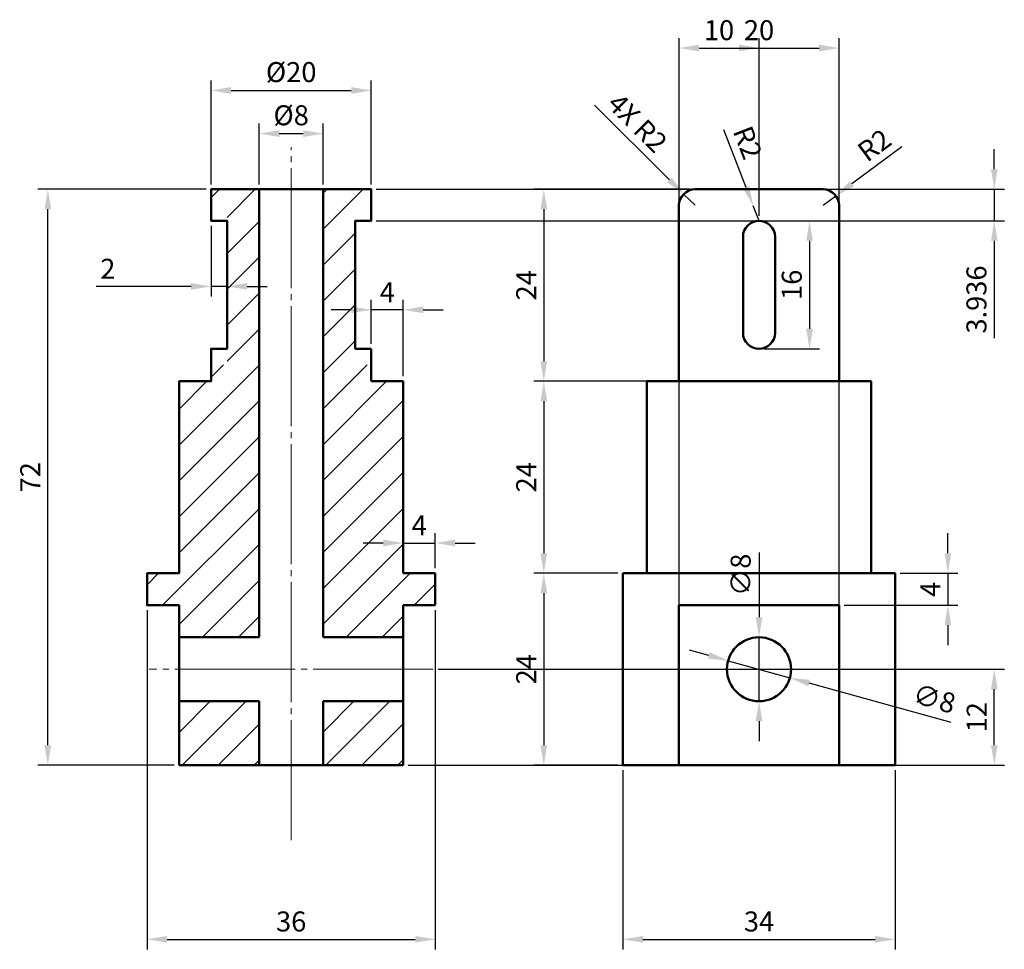
# Model space of a CAD drawing. Units: millimetres. Extents: x 2656 to 2779, y 1429 to 1546.
import ezdxf

# ---------------------------------------------------------------- set-up
doc = ezdxf.new("R2010")
doc.units = ezdxf.units.MM
doc.linetypes.add('JIS_08_15', pattern=[17.25, 15, -0.75, 0.75, -0.75])
for name, color, linetype, lineweight in [('M-CNTR', 1, 'JIS_08_15', 18), ('M-DIMS', 2, 'Continuous', 25), ('M-HATC', 8, 'Continuous', 18), ('M-OUTL', 7, 'Continuous', 50)]:
    doc.layers.add(name, color=color, linetype=linetype, lineweight=lineweight)
doc.styles.get("Standard").update_dxf_attribs({"font": 'arial.ttf'})
doc.dimstyles.new('ISO-25', dxfattribs={"dimtxt": 2.5, "dimasz": 2.5, "dimexe": 1.25, "dimexo": 0.625, "dimtad": 1, "dimdec": 0, "dimtxsty": 'Standard', "dimcen": 2.5, "dimadec": 0, "dimazin": 0, "dimtfac": 1, "dimtdec": 0, "dimtmove": 0, "dimatfit": 3, "dimfxl": 1, "dimarcsym": 0})

# ---------------------------------------------------------------- blocks, each defined once
blk = doc.blocks.new('*D4')
at = {"layer": 'Defpoints', "color": 0, "transparency": 16777216}
for p in [(2700.11, 1536.86), (2680.11, 1524.5), (2700.11, 1524.5)]:
    blk.add_point(p, dxfattribs=at)
at = {"layer": 'M-DIMS', "color": 0, "lineweight": -2, "transparency": 16777216}
for p, q in [((2680.11, 1525.12), (2680.11, 1538.11)), ((2700.11, 1525.12), (2700.11, 1538.11)), ((2682.61, 1536.86), (2697.61, 1536.86))]:
    blk.add_line(p, q, dxfattribs=at)
at = {"layer": 'M-DIMS', "color": 0, "transparency": 16777216}
for points in [[(2682.61, 1537.28), (2682.61, 1536.44), (2680.11, 1536.86)], [(2697.61, 1537.28), (2697.61, 1536.44), (2700.11, 1536.86)]]:
    blk.add_solid(points, dxfattribs=at)
at = {"layer": 'M-DIMS', "color": 0, "transparency": 16777216, "insert": (2690.11, 1538.83), "char_height": 2.5, "attachment_point": 5}
blk.add_mtext('%%C20', dxfattribs=at)
blk = doc.blocks.new('*D5')
at = {"layer": 'Defpoints', "color": 0, "transparency": 16777216}
for p in [(2694.11, 1531.46), (2686.11, 1524.5), (2694.11, 1524.5)]:
    blk.add_point(p, dxfattribs=at)
at = {"layer": 'M-DIMS', "color": 0, "lineweight": -2, "transparency": 16777216}
for p, q in [((2686.11, 1525.12), (2686.11, 1532.71)), ((2694.11, 1525.12), (2694.11, 1532.71)), ((2688.61, 1531.46), (2691.61, 1531.46))]:
    blk.add_line(p, q, dxfattribs=at)
at = {"layer": 'M-DIMS', "color": 0, "transparency": 16777216}
for points in [[(2688.61, 1531.87), (2688.61, 1531.04), (2686.11, 1531.46)], [(2691.61, 1531.87), (2691.61, 1531.04), (2694.11, 1531.46)]]:
    blk.add_solid(points, dxfattribs=at)
at = {"layer": 'M-DIMS', "color": 0, "transparency": 16777216, "insert": (2690.11, 1533.43), "char_height": 2.5, "attachment_point": 5}
blk.add_mtext('%%C8', dxfattribs=at)
blk = doc.blocks.new('*D6')
at = {"layer": 'Defpoints', "color": 0, "transparency": 16777216}
for p in [(2680.11, 1520.56), (2682.11, 1520.56), (2682.11, 1512.36)]:
    blk.add_point(p, dxfattribs=at)
at = {"layer": 'M-DIMS', "color": 0, "lineweight": -2, "transparency": 16777216}
for p, q in [((2680.11, 1519.94), (2680.11, 1511.11)), ((2682.11, 1519.94), (2682.11, 1511.11)), ((2677.61, 1512.36), (2665.75, 1512.36)), ((2682.11, 1512.36), (2680.11, 1512.36)), ((2684.61, 1512.36), (2687.11, 1512.36))]:
    blk.add_line(p, q, dxfattribs=at)
at = {"layer": 'M-DIMS', "color": 0, "transparency": 16777216}
for points in [[(2677.61, 1512.78), (2677.61, 1511.95), (2680.11, 1512.36)], [(2684.61, 1512.78), (2684.61, 1511.95), (2682.11, 1512.36)]]:
    blk.add_solid(points, dxfattribs=at)
at = {"layer": 'M-DIMS', "color": 0, "transparency": 16777216, "insert": (2667.2, 1514.24), "char_height": 2.5, "attachment_point": 5}
blk.add_mtext('2', dxfattribs=at)
blk = doc.blocks.new('*D7')
at = {"layer": 'Defpoints', "color": 0, "transparency": 16777216}
for p in [(2708.11, 1480.28), (2704.11, 1476.5), (2708.11, 1476.5)]:
    blk.add_point(p, dxfattribs=at)
at = {"layer": 'M-DIMS', "color": 0, "lineweight": -2, "transparency": 16777216}
for p, q in [((2704.11, 1477.12), (2704.11, 1481.53)), ((2708.11, 1477.12), (2708.11, 1481.53)), ((2701.61, 1480.28), (2699.11, 1480.28)), ((2704.11, 1480.28), (2708.11, 1480.28)), ((2710.61, 1480.28), (2713.11, 1480.28))]:
    blk.add_line(p, q, dxfattribs=at)
at = {"layer": 'M-DIMS', "color": 0, "transparency": 16777216}
for points in [[(2701.61, 1480.7), (2701.61, 1479.86), (2704.11, 1480.28)], [(2710.61, 1480.7), (2710.61, 1479.86), (2708.11, 1480.28)]]:
    blk.add_solid(points, dxfattribs=at)
at = {"layer": 'M-DIMS', "color": 0, "transparency": 16777216, "insert": (2706.11, 1482.16), "char_height": 2.5, "attachment_point": 5}
blk.add_mtext('4', dxfattribs=at)
blk = doc.blocks.new('*D8')
at = {"layer": 'Defpoints', "color": 0, "transparency": 16777216}
for p in [(2758.17, 1523.69), (2756.57, 1522.5)]:
    blk.add_point(p, dxfattribs=at)
at = {"layer": 'M-DIMS', "color": 0, "lineweight": -2, "transparency": 16777216}
for p, q in [((2766.4, 1529.81), (2760.18, 1525.18)), ((2756.57, 1522.5), (2758.17, 1523.69))]:
    blk.add_line(p, q, dxfattribs=at)
at = {"layer": 'M-DIMS', "color": 0, "transparency": 16777216}
blk.add_solid([(2759.93, 1525.52), (2760.43, 1524.85), (2758.17, 1523.69)], dxfattribs=at)
at = {"layer": 'M-DIMS', "color": 0, "transparency": 16777216, "insert": (2763.17, 1529.75), "char_height": 2.5, "attachment_point": 5, "rotation": 36.6494}
blk.add_mtext('R2', dxfattribs=at)
blk = doc.blocks.new('*D1')
at = {"layer": 'Defpoints', "color": 0, "transparency": 16777216}
for p in [(2747.85, 1522.43), (2748.57, 1520.56)]:
    blk.add_point(p, dxfattribs=at)
at = {"layer": 'M-DIMS', "color": 0, "lineweight": -2, "transparency": 16777216}
for p, q in [((2744.15, 1531.99), (2746.94, 1524.76)), ((2748.57, 1520.56), (2747.85, 1522.43))]:
    blk.add_line(p, q, dxfattribs=at)
at = {"layer": 'M-DIMS', "color": 0, "transparency": 16777216}
blk.add_solid([(2747.33, 1524.91), (2746.56, 1524.61), (2747.85, 1522.43)], dxfattribs=at)
at = {"layer": 'M-DIMS', "color": 0, "transparency": 16777216, "insert": (2746.85, 1530.22), "char_height": 2.5, "attachment_point": 5, "rotation": 291.129}
blk.add_mtext('R2', dxfattribs=at)
blk = doc.blocks.new('*D2')
at = {"layer": 'Defpoints', "color": 0, "transparency": 16777216}
for p in [(2748.57, 1520.56), (2748.57, 1504.56), (2754.88, 1504.56)]:
    blk.add_point(p, dxfattribs=at)
at = {"layer": 'M-DIMS', "color": 0, "lineweight": -2, "transparency": 16777216}
for p, q in [((2749.19, 1520.56), (2756.13, 1520.56)), ((2754.88, 1518.06), (2754.88, 1507.06)), ((2749.19, 1504.56), (2756.13, 1504.56))]:
    blk.add_line(p, q, dxfattribs=at)
at = {"layer": 'M-DIMS', "color": 0, "transparency": 16777216}
for points in [[(2754.46, 1518.06), (2755.3, 1518.06), (2754.88, 1520.56)], [(2754.46, 1507.06), (2755.3, 1507.06), (2754.88, 1504.56)]]:
    blk.add_solid(points, dxfattribs=at)
at = {"layer": 'M-DIMS', "color": 0, "transparency": 16777216, "insert": (2752.98, 1512.56), "char_height": 2.5, "attachment_point": 5, "rotation": 90}
blk.add_mtext('16', dxfattribs=at)
blk = doc.blocks.new('*D9')
at = {"layer": 'Defpoints', "color": 0, "transparency": 16777216}
for p in [(2740.57, 1524.5), (2721.68, 1500.5), (2738.57, 1500.5)]:
    blk.add_point(p, dxfattribs=at)
at = {"layer": 'M-DIMS', "color": 0, "lineweight": -2, "transparency": 16777216}
for p, q in [((2739.94, 1524.5), (2720.43, 1524.5)), ((2721.68, 1522), (2721.68, 1503)), ((2737.94, 1500.5), (2720.43, 1500.5))]:
    blk.add_line(p, q, dxfattribs=at)
at = {"layer": 'M-DIMS', "color": 0, "transparency": 16777216}
for points in [[(2721.26, 1522), (2722.1, 1522), (2721.68, 1524.5)], [(2721.26, 1503), (2722.1, 1503), (2721.68, 1500.5)]]:
    blk.add_solid(points, dxfattribs=at)
at = {"layer": 'M-DIMS', "color": 0, "transparency": 16777216, "insert": (2719.8, 1512.5), "char_height": 2.5, "attachment_point": 5, "rotation": 90}
blk.add_mtext('24', dxfattribs=at)
blk = doc.blocks.new('*D10')
at = {"layer": 'Defpoints', "color": 0, "transparency": 16777216}
for p in [(2734.57, 1500.5), (2721.68, 1476.5), (2731.57, 1476.5)]:
    blk.add_point(p, dxfattribs=at)
at = {"layer": 'M-DIMS', "color": 0, "lineweight": -2, "transparency": 16777216}
for p, q in [((2733.94, 1500.5), (2720.43, 1500.5)), ((2721.68, 1498), (2721.68, 1479)), ((2730.94, 1476.5), (2720.43, 1476.5))]:
    blk.add_line(p, q, dxfattribs=at)
at = {"layer": 'M-DIMS', "color": 0, "transparency": 16777216}
for points in [[(2721.26, 1498), (2722.1, 1498), (2721.68, 1500.5)], [(2721.26, 1479), (2722.1, 1479), (2721.68, 1476.5)]]:
    blk.add_solid(points, dxfattribs=at)
at = {"layer": 'M-DIMS', "color": 0, "transparency": 16777216, "insert": (2719.8, 1488.5), "char_height": 2.5, "attachment_point": 5, "rotation": 90}
blk.add_mtext('24', dxfattribs=at)
blk = doc.blocks.new('*D3')
at = {"layer": 'Defpoints', "color": 0, "transparency": 16777216}
for p in [(2731.57, 1476.5), (2721.68, 1452.5), (2731.57, 1452.5)]:
    blk.add_point(p, dxfattribs=at)
at = {"layer": 'M-DIMS', "color": 0, "lineweight": -2, "transparency": 16777216}
for p, q in [((2730.94, 1476.5), (2720.43, 1476.5)), ((2721.68, 1474), (2721.68, 1455)), ((2730.94, 1452.5), (2720.43, 1452.5))]:
    blk.add_line(p, q, dxfattribs=at)
at = {"layer": 'M-DIMS', "color": 0, "transparency": 16777216}
for points in [[(2721.26, 1474), (2722.1, 1474), (2721.68, 1476.5)], [(2721.26, 1455), (2722.1, 1455), (2721.68, 1452.5)]]:
    blk.add_solid(points, dxfattribs=at)
at = {"layer": 'M-DIMS', "color": 0, "transparency": 16777216, "insert": (2719.8, 1464.5), "char_height": 2.5, "attachment_point": 5, "rotation": 90}
blk.add_mtext('24', dxfattribs=at)
blk = doc.blocks.new('*D11')
at = {"layer": 'Defpoints', "color": 0, "transparency": 16777216}
for p in [(2765.57, 1476.5), (2758.57, 1472.5), (2772.17, 1472.5)]:
    blk.add_point(p, dxfattribs=at)
at = {"layer": 'M-DIMS', "color": 0, "lineweight": -2, "transparency": 16777216}
for p, q in [((2772.17, 1479), (2772.17, 1481.5)), ((2766.19, 1476.5), (2773.42, 1476.5)), ((2772.17, 1476.5), (2772.17, 1472.5)), ((2759.19, 1472.5), (2773.42, 1472.5)), ((2772.17, 1470), (2772.17, 1467.5))]:
    blk.add_line(p, q, dxfattribs=at)
at = {"layer": 'M-DIMS', "color": 0, "transparency": 16777216}
for points in [[(2771.76, 1479), (2772.59, 1479), (2772.17, 1476.5)], [(2771.76, 1470), (2772.59, 1470), (2772.17, 1472.5)]]:
    blk.add_solid(points, dxfattribs=at)
at = {"layer": 'M-DIMS', "color": 0, "transparency": 16777216, "insert": (2770.3, 1474.5), "char_height": 2.5, "attachment_point": 5, "rotation": 90}
blk.add_mtext('4', dxfattribs=at)
blk = doc.blocks.new('*D12')
at = {"layer": 'Defpoints', "color": 0, "transparency": 16777216}
for p in [(2744.71, 1465.56), (2752.42, 1463.43)]:
    blk.add_point(p, dxfattribs=at)
at = {"layer": 'M-DIMS', "color": 0, "lineweight": -2, "transparency": 16777216}
for p, q in [((2742.3, 1466.23), (2739.89, 1466.9)), ((2744.71, 1465.56), (2752.42, 1463.43)), ((2772.57, 1457.86), (2754.83, 1462.76))]:
    blk.add_line(p, q, dxfattribs=at)
at = {"layer": 'M-DIMS', "color": 0, "transparency": 16777216}
for points in [[(2742.41, 1466.63), (2742.19, 1465.83), (2744.71, 1465.56)], [(2754.94, 1463.17), (2754.72, 1462.36), (2752.42, 1463.43)]]:
    blk.add_solid(points, dxfattribs=at)
at = {"layer": 'M-DIMS', "color": 0, "transparency": 16777216, "insert": (2770.39, 1460.51), "char_height": 2.5, "attachment_point": 5, "rotation": 344.5424}
blk.add_mtext('∅8', dxfattribs=at)
blk = doc.blocks.new('*D13')
at = {"layer": 'Defpoints', "color": 0, "transparency": 16777216}
for p in [(2700.11, 1509.43), (2700.11, 1504.56), (2704.11, 1500.5)]:
    blk.add_point(p, dxfattribs=at)
at = {"layer": 'M-DIMS', "color": 0, "lineweight": -2, "transparency": 16777216}
for p, q in [((2700.11, 1505.19), (2700.11, 1510.68)), ((2704.11, 1501.12), (2704.11, 1510.68)), ((2697.61, 1509.43), (2695.11, 1509.43)), ((2704.11, 1509.43), (2700.11, 1509.43)), ((2706.61, 1509.43), (2709.11, 1509.43))]:
    blk.add_line(p, q, dxfattribs=at)
at = {"layer": 'M-DIMS', "color": 0, "transparency": 16777216}
for points in [[(2697.61, 1509.85), (2697.61, 1509.02), (2700.11, 1509.43)], [(2706.61, 1509.85), (2706.61, 1509.02), (2704.11, 1509.43)]]:
    blk.add_solid(points, dxfattribs=at)
at = {"layer": 'M-DIMS', "color": 0, "transparency": 16777216, "insert": (2702.11, 1511.31), "char_height": 2.5, "attachment_point": 5}
blk.add_mtext('4', dxfattribs=at)
blk = doc.blocks.new('*D14')
at = {"layer": 'Defpoints', "color": 0, "transparency": 16777216}
for p in [(2672.11, 1472.5), (2708.11, 1472.5), (2708.11, 1430.73)]:
    blk.add_point(p, dxfattribs=at)
at = {"layer": 'M-DIMS', "color": 0, "lineweight": -2, "transparency": 16777216}
for p, q in [((2672.11, 1471.87), (2672.11, 1429.48)), ((2708.11, 1471.87), (2708.11, 1429.48)), ((2674.61, 1430.73), (2705.61, 1430.73))]:
    blk.add_line(p, q, dxfattribs=at)
at = {"layer": 'M-DIMS', "color": 0, "transparency": 16777216}
for points in [[(2674.61, 1431.15), (2674.61, 1430.32), (2672.11, 1430.73)], [(2705.61, 1431.15), (2705.61, 1430.32), (2708.11, 1430.73)]]:
    blk.add_solid(points, dxfattribs=at)
at = {"layer": 'M-DIMS', "color": 0, "transparency": 16777216, "insert": (2690.11, 1432.64), "char_height": 2.5, "attachment_point": 5}
blk.add_mtext('36', dxfattribs=at)
blk = doc.blocks.new('*D15')
at = {"layer": 'Defpoints', "color": 0, "transparency": 16777216}
for p in [(2731.57, 1452.5), (2765.57, 1452.5), (2765.57, 1430.73)]:
    blk.add_point(p, dxfattribs=at)
at = {"layer": 'M-DIMS', "color": 0, "lineweight": -2, "transparency": 16777216}
for p, q in [((2731.57, 1451.87), (2731.57, 1429.48)), ((2765.57, 1451.87), (2765.57, 1429.48)), ((2734.07, 1430.73), (2763.07, 1430.73))]:
    blk.add_line(p, q, dxfattribs=at)
at = {"layer": 'M-DIMS', "color": 0, "transparency": 16777216}
for points in [[(2734.07, 1431.15), (2734.07, 1430.32), (2731.57, 1430.73)], [(2763.07, 1431.15), (2763.07, 1430.32), (2765.57, 1430.73)]]:
    blk.add_solid(points, dxfattribs=at)
at = {"layer": 'M-DIMS', "color": 0, "transparency": 16777216, "insert": (2748.57, 1432.64), "char_height": 2.5, "attachment_point": 5}
blk.add_mtext('34', dxfattribs=at)
blk = doc.blocks.new('*D16')
at = {"layer": 'Defpoints', "color": 0, "transparency": 16777216}
for p in [(2659.71, 1524.5), (2680.11, 1524.5), (2676.11, 1452.5)]:
    blk.add_point(p, dxfattribs=at)
at = {"layer": 'M-DIMS', "color": 0, "lineweight": -2, "transparency": 16777216}
for p, q in [((2679.48, 1524.5), (2658.46, 1524.5)), ((2659.71, 1455), (2659.71, 1522)), ((2675.48, 1452.5), (2658.46, 1452.5))]:
    blk.add_line(p, q, dxfattribs=at)
at = {"layer": 'M-DIMS', "color": 0, "transparency": 16777216}
for points in [[(2659.29, 1522), (2660.12, 1522), (2659.71, 1524.5)], [(2659.29, 1455), (2660.12, 1455), (2659.71, 1452.5)]]:
    blk.add_solid(points, dxfattribs=at)
at = {"layer": 'M-DIMS', "color": 0, "transparency": 16777216, "insert": (2657.83, 1488.5), "char_height": 2.5, "attachment_point": 5, "rotation": 90}
blk.add_mtext('72', dxfattribs=at)
blk = doc.blocks.new('*D17')
at = {"layer": 'Defpoints', "color": 0, "transparency": 16777216}
for p in [(2707.84, 1464.5), (2777.97, 1464.5), (2704.11, 1452.5)]:
    blk.add_point(p, dxfattribs=at)
at = {"layer": 'M-DIMS', "color": 0, "lineweight": -2, "transparency": 16777216}
for p, q in [((2708.46, 1464.5), (2779.22, 1464.5)), ((2777.97, 1455), (2777.97, 1462)), ((2704.73, 1452.5), (2779.22, 1452.5))]:
    blk.add_line(p, q, dxfattribs=at)
at = {"layer": 'M-DIMS', "color": 0, "transparency": 16777216}
for points in [[(2777.55, 1462), (2778.38, 1462), (2777.97, 1464.5)], [(2777.55, 1455), (2778.38, 1455), (2777.97, 1452.5)]]:
    blk.add_solid(points, dxfattribs=at)
at = {"layer": 'M-DIMS', "color": 0, "transparency": 16777216, "insert": (2776.09, 1458.5), "char_height": 2.5, "attachment_point": 5, "rotation": 90}
blk.add_mtext('12', dxfattribs=at)
blk = doc.blocks.new('*D18')
at = {"layer": 'Defpoints', "color": 0, "transparency": 16777216}
for p in [(2700.11, 1524.5), (2700.11, 1520.56), (2777.97, 1520.56)]:
    blk.add_point(p, dxfattribs=at)
at = {"layer": 'M-DIMS', "color": 0, "lineweight": -2, "transparency": 16777216}
for p, q in [((2777.97, 1527), (2777.97, 1529.5)), ((2700.73, 1524.5), (2779.22, 1524.5)), ((2777.97, 1524.5), (2777.97, 1520.56)), ((2700.73, 1520.56), (2779.22, 1520.56)), ((2777.97, 1518.06), (2777.97, 1505.88))]:
    blk.add_line(p, q, dxfattribs=at)
at = {"layer": 'M-DIMS', "color": 0, "transparency": 16777216}
for points in [[(2777.55, 1527), (2778.38, 1527), (2777.97, 1524.5)], [(2777.55, 1518.06), (2778.38, 1518.06), (2777.97, 1520.56)]]:
    blk.add_solid(points, dxfattribs=at)
at = {"layer": 'M-DIMS', "color": 0, "transparency": 16777216, "insert": (2776.06, 1510.72), "char_height": 2.5, "attachment_point": 5, "rotation": 90}
blk.add_mtext('3.936', dxfattribs=at)
blk = doc.blocks.new('*D19')
at = {"layer": 'Defpoints', "color": 0, "transparency": 16777216}
for p in [(2758.57, 1542.16), (2738.57, 1452.5), (2758.57, 1452.5)]:
    blk.add_point(p, dxfattribs=at)
at = {"layer": 'M-DIMS', "color": 0, "lineweight": -2, "transparency": 16777216}
for p, q in [((2738.57, 1453.12), (2738.57, 1543.41)), ((2758.57, 1453.12), (2758.57, 1543.41)), ((2741.07, 1542.16), (2756.07, 1542.16))]:
    blk.add_line(p, q, dxfattribs=at)
at = {"layer": 'M-DIMS', "color": 0, "transparency": 16777216}
for points in [[(2741.07, 1542.58), (2741.07, 1541.75), (2738.57, 1542.16)], [(2756.07, 1542.58), (2756.07, 1541.75), (2758.57, 1542.16)]]:
    blk.add_solid(points, dxfattribs=at)
at = {"layer": 'M-DIMS', "color": 0, "transparency": 16777216, "insert": (2748.57, 1544.07), "char_height": 2.5, "attachment_point": 5}
blk.add_mtext('20', dxfattribs=at)
blk = doc.blocks.new('*D20')
at = {"layer": 'Defpoints', "color": 0, "transparency": 16777216}
for p in [(2748.57, 1542.16), (2738.57, 1522.5), (2748.57, 1520.56)]:
    blk.add_point(p, dxfattribs=at)
at = {"layer": 'M-DIMS', "color": 0, "lineweight": -2, "transparency": 16777216}
for p, q in [((2738.57, 1523.12), (2738.57, 1543.41)), ((2748.57, 1521.19), (2748.57, 1543.41)), ((2741.07, 1542.16), (2746.07, 1542.16))]:
    blk.add_line(p, q, dxfattribs=at)
at = {"layer": 'M-DIMS', "color": 0, "transparency": 16777216}
for points in [[(2741.07, 1542.58), (2741.07, 1541.75), (2738.57, 1542.16)], [(2746.07, 1542.58), (2746.07, 1541.75), (2748.57, 1542.16)]]:
    blk.add_solid(points, dxfattribs=at)
at = {"layer": 'M-DIMS', "color": 0, "transparency": 16777216, "insert": (2743.57, 1544.07), "char_height": 2.5, "attachment_point": 5}
blk.add_mtext('10', dxfattribs=at)
blk = doc.blocks.new('*D21')
at = {"layer": 'Defpoints', "color": 0, "transparency": 16777216}
for p in [(2748.57, 1468.5), (2748.57, 1460.5)]:
    blk.add_point(p, dxfattribs=at)
at = {"layer": 'M-DIMS', "color": 0, "lineweight": -2, "transparency": 16777216}
for p, q in [((2748.57, 1479.11), (2748.57, 1471)), ((2748.57, 1460.5), (2748.57, 1468.5)), ((2748.57, 1458), (2748.57, 1455.5))]:
    blk.add_line(p, q, dxfattribs=at)
at = {"layer": 'M-DIMS', "color": 0, "transparency": 16777216}
for points in [[(2748.15, 1471), (2748.98, 1471), (2748.57, 1468.5)], [(2748.15, 1458), (2748.98, 1458), (2748.57, 1460.5)]]:
    blk.add_solid(points, dxfattribs=at)
at = {"layer": 'M-DIMS', "color": 0, "transparency": 16777216, "insert": (2746.6, 1476.3), "char_height": 2.5, "attachment_point": 5, "rotation": 89.9948}
blk.add_mtext('∅8', dxfattribs=at)
blk = doc.blocks.new('*D22')
at = {"layer": 'Defpoints', "color": 0, "transparency": 16777216}
for p in [(2739.15, 1523.91), (2740.57, 1522.5)]:
    blk.add_point(p, dxfattribs=at)
at = {"layer": 'M-DIMS', "color": 0, "lineweight": -2, "transparency": 16777216}
for p, q in [((2728.03, 1535.03), (2737.38, 1525.68)), ((2740.57, 1522.5), (2739.15, 1523.91))]:
    blk.add_line(p, q, dxfattribs=at)
at = {"layer": 'M-DIMS', "color": 0, "transparency": 16777216}
blk.add_solid([(2737.68, 1525.97), (2737.09, 1525.38), (2739.15, 1523.91)], dxfattribs=at)
at = {"layer": 'M-DIMS', "color": 0, "transparency": 16777216, "insert": (2733.15, 1532.57), "char_height": 2.5, "attachment_point": 5, "rotation": 315.0103}
blk.add_mtext('4X R2', dxfattribs=at)

msp = doc.modelspace()

# ---------------------------------------------------------------- hatches: boundary and pattern name
at = {"layer": 'M-HATC'}
h = msp.add_hatch(dxfattribs=at)
h.set_pattern_fill('ANSI31', color=256)
h.set_pattern_definition([(45, (-1079.2516, -4.2968), (-2.245064, 2.245064), [])])
h.paths.add_polyline_path([(2686.1081, 1524.4969), (2680.1081, 1524.4969), (2680.1081, 1522.5607), (2682.1081, 1522.5607), (2682.1081, 1502.5607), (2680.1081, 1502.5607), (2680.1081, 1500.4969), (2676.1081, 1500.4969), (2676.1081, 1476.4969), (2672.1081, 1476.4969), (2672.1081, 1472.4969), (2676.1081, 1472.4969), (2676.1081, 1468.4969), (2686.1081, 1468.4969)])
h.paths.add_polyline_path([(2704.1081, 1500.4969), (2700.1081, 1500.4969), (2700.1081, 1502.5607), (2698.1081, 1502.5607), (2698.1081, 1522.5607), (2700.1081, 1522.5607), (2700.1081, 1524.4969), (2694.1081, 1524.4969), (2694.1081, 1468.4969), (2704.1081, 1468.4969), (2704.1081, 1472.4969), (2708.1081, 1472.4969), (2708.1081, 1476.4969), (2704.1081, 1476.4969)])
h.paths.add_polyline_path([(2704.1081, 1460.4969), (2694.1081, 1460.4969), (2694.1081, 1452.4969), (2704.1081, 1452.4969)])
h.paths.add_polyline_path([(2686.1081, 1460.4969), (2676.1081, 1460.4969), (2676.1081, 1452.4969), (2686.1081, 1452.4969)])

# ---------------------------------------------------------------- linework, layer by layer
at = {"layer": 'M-CNTR'}
for p, q in [((2690.1081, 1443.1327), (2690.1081, 1529.7636)), ((2707.8385, 1464.4969), (2672.3777, 1464.4969))]:
    msp.add_line(p, q, dxfattribs=at)
at = {"layer": 'M-OUTL'}
for p, q in [((2686.1081, 1524.4969), (2686.1081, 1468.4969)), ((2694.1081, 1524.4969), (2694.1081, 1468.4969)), ((2746.5666, 1518.5607), (2746.5666, 1506.5607)), ((2750.5666, 1506.5607), (2750.5666, 1518.5607)), ((2698.1081, 1504.5607), (2700.1081, 1504.5607)), ((2700.1081, 1504.5607), (2700.1081, 1500.4969)), ((2700.1081, 1500.4969), (2704.1081, 1500.4969)), ((2704.1081, 1500.4969), (2704.1081, 1476.4969)), ((2704.1081, 1476.4969), (2708.1081, 1476.4969)), ((2708.1081, 1476.4969), (2708.1081, 1472.4969)), ((2708.1081, 1472.4969), (2704.1081, 1472.4969)), ((2704.1081, 1472.4969), (2704.1081, 1452.4969)), ((2686.1081, 1468.4969), (2676.1081, 1468.4969)), ((2704.1081, 1468.4969), (2694.1081, 1468.4969)), ((2686.1081, 1460.4969), (2676.1081, 1460.4969)), ((2686.1081, 1460.4969), (2686.1081, 1452.4969)), ((2694.1081, 1460.4969), (2694.1081, 1452.4969)), ((2704.1081, 1460.4969), (2694.1081, 1460.4969)), ((2704.1081, 1452.4969), (2676.1081, 1452.4969))]:
    msp.add_line(p, q, dxfattribs=at)
for points in [[(2698.1081, 1504.5607), (2698.1081, 1520.5607), (2700.1081, 1520.5607), (2700.1081, 1524.4969), (2680.1081, 1524.4969), (2680.1081, 1520.5607), (2682.1081, 1520.5607), (2682.1081, 1504.5607)], [(2680.1081, 1504.5607), (2682.1081, 1504.5607), (2680.1081, 1504.5607), (2680.1081, 1500.4969), (2676.1081, 1500.4969), (2676.1081, 1476.4969), (2672.1081, 1476.4969), (2672.1081, 1472.4969), (2676.1081, 1472.4969), (2676.1081, 1452.4969)]]:
    msp.add_lwpolyline(points, dxfattribs=at)
msp.add_lwpolyline([(2740.5666, 1524.4969), (2756.5666, 1524.4969, -0.41421356), (2758.5666, 1522.4969), (2758.5666, 1500.4969), (2738.5666, 1500.4969), (2738.5666, 1522.4969, -0.41421356)], format="xyb", close=True, dxfattribs=at)
for points in [[(2734.5666, 1500.4969), (2762.5666, 1500.4969), (2762.5666, 1476.4969), (2734.5666, 1476.4969)], [(2731.5666, 1476.4969), (2765.5666, 1476.4969), (2765.5666, 1452.4969), (2731.5666, 1452.4969)], [(2738.5666, 1472.4969), (2758.5666, 1472.4969), (2758.5666, 1452.4969), (2738.5666, 1452.4969)]]:
    msp.add_lwpolyline(points, close=True, dxfattribs=at)
msp.add_circle((2748.5666, 1464.4969), 4, dxfattribs=at)
for centre, start, end in [((2748.5666, 1518.5607), 0, 180), ((2748.5666, 1506.5607), 180, 0)]:
    msp.add_arc(centre, 2, start, end, dxfattribs=at)

# ---------------------------------------------------------------- dimensions: what is measured, and where the dimension line sits
at = {"layer": 'M-DIMS'}
for base, p1, p2, override, picture, middle in [((2758.5666, 1542.1636), (2738.5666, 1452.4969), (2758.5666, 1452.4969), {"dimdec": 0, "dimlfac": 1, "dimrnd": 0, "dimzin": 0, "dimdsep": 46, "dimlunit": 2}, '*D19', (2748.5666, 1544.065)), ((2748.5666, 1542.1636), (2738.5666, 1522.4969), (2748.5666, 1520.5607), {"dimdec": 0, "dimlfac": 1, "dimrnd": 0, "dimzin": 0, "dimdsep": 46, "dimlunit": 2}, '*D20', (2743.5666, 1544.065)), ((2700.1081, 1509.4332), (2704.1081, 1500.4969), (2700.1081, 1504.5607), {"dimclrd": 0, "dimclre": 0, "dimclrt": 0}, '*D13', (2702.1081, 1511.3082)), ((2708.1081, 1480.2812), (2704.1081, 1476.4969), (2708.1081, 1476.4969), {"dimclrd": 0, "dimclre": 0, "dimclrt": 0}, '*D7', (2706.1081, 1482.1562)), ((2708.1081, 1430.7327), (2672.1081, 1472.4969), (2708.1081, 1472.4969), {"dimdec": 0, "dimlfac": 1, "dimrnd": 0, "dimzin": 0, "dimdsep": 46, "dimlunit": 2}, '*D14', (2690.1081, 1432.635)), ((2765.5666, 1430.7327), (2731.5666, 1452.4969), (2765.5666, 1452.4969), {"dimdec": 0, "dimlfac": 1, "dimrnd": 0, "dimzin": 0, "dimdsep": 46, "dimlunit": 2}, '*D15', (2748.5666, 1432.635))]:
    dim = msp.add_linear_dim(base=base, p1=p1, p2=p2, dimstyle='ISO-25', override=override, dxfattribs=at)
    dim.commit()
    dim.dimension.update_dxf_attribs({"geometry": picture, "text_midpoint": middle})
for base, p1, p2, picture, middle in [((2700.1081, 1536.8595), (2680.1081, 1524.4969), (2700.1081, 1524.4969), '*D4', (2690.1081, 1538.8309)), ((2694.1081, 1531.458), (2686.1081, 1524.4969), (2694.1081, 1524.4969), '*D5', (2690.1081, 1533.4294))]:
    dim = msp.add_linear_dim(base=base, p1=p1, p2=p2, text='%%C<>', dimstyle='ISO-25', override={"dimclrd": 0, "dimclre": 0, "dimclrt": 0}, dxfattribs=at)
    dim.commit()
    dim.dimension.update_dxf_attribs({"geometry": picture, "text_midpoint": middle})
dim = msp.add_radius_dim(center=(2740.5666, 1522.4969), mpoint=(2739.1522, 1523.9108), text='4X <>', dimstyle='ISO-25', override={"dimdec": 0, "dimlfac": 1, "dimrnd": 0, "dimzin": 0, "dimdsep": 46, "dimlunit": 2}, dxfattribs=at)
dim.commit()
dim.dimension.update_dxf_attribs({"geometry": '*D22', "text_midpoint": (2733.1522, 1532.5683)})
for center, mpoint, picture, middle in [((2748.5666, 1520.5607), (2747.8457, 1522.4263), '*D1', (2746.8498, 1530.2191)), ((2756.5666, 1522.4969), (2758.1712, 1523.6907), '*D8', (2763.1689, 1529.7523))]:
    dim = msp.add_radius_dim(center=center, mpoint=mpoint, dimstyle='ISO-25', override={"dimclrd": 0, "dimclre": 0, "dimclrt": 0}, dxfattribs=at)
    dim.commit()
    dim.dimension.update_dxf_attribs({"geometry": picture, "text_midpoint": middle})
for base, p1, p2, override, picture, middle in [((2777.9666, 1520.5607), (2700.1081, 1524.4969), (2700.1081, 1520.5607), {"dimdec": 3, "dimlfac": 1, "dimrnd": 0, "dimzin": 0, "dimdsep": 46, "dimlunit": 2}, '*D18', (2776.0644, 1510.7193)), ((2659.7081, 1524.4969), (2676.1081, 1452.4969), (2680.1081, 1524.4969), {"dimdec": 0, "dimlfac": 1, "dimrnd": 0, "dimzin": 0, "dimdsep": 46, "dimlunit": 2}, '*D16', (2657.828, 1488.4969)), ((2721.6792, 1500.4969), (2740.5666, 1524.4969), (2738.5666, 1500.4969), {"dimclrd": 0, "dimclre": 0, "dimclrt": 0}, '*D9', (2719.7991, 1512.4969)), ((2754.8812, 1504.5607), (2748.5666, 1520.5607), (2748.5666, 1504.5607), {"dimclrd": 0, "dimclre": 0, "dimclrt": 0}, '*D2', (2752.9798, 1512.5607)), ((2721.6792, 1476.4969), (2734.5666, 1500.4969), (2731.5666, 1476.4969), {"dimclrd": 0, "dimclre": 0, "dimclrt": 0}, '*D10', (2719.7991, 1488.4969)), ((2772.1735, 1472.4969), (2765.5666, 1476.4969), (2758.5666, 1472.4969), {"dimclrd": 0, "dimclre": 0, "dimclrt": 0}, '*D11', (2770.2985, 1474.4969)), ((2721.6792, 1452.4969), (2731.5666, 1476.4969), (2731.5666, 1452.4969), {"dimclrd": 0, "dimclre": 0, "dimclrt": 0}, '*D3', (2719.7991, 1464.4969)), ((2777.9666, 1464.4969), (2704.1081, 1452.4969), (2707.8385, 1464.4969), {"dimdec": 0, "dimlfac": 1, "dimrnd": 0, "dimzin": 0, "dimdsep": 46, "dimlunit": 2}, '*D17', (2776.0865, 1458.4969))]:
    dim = msp.add_linear_dim(base=base, p1=p1, p2=p2, angle=90, dimstyle='ISO-25', override=override, dxfattribs=at)
    dim.commit()
    dim.dimension.update_dxf_attribs({"geometry": picture, "text_midpoint": middle})
dim = msp.add_linear_dim(base=(2682.1081, 1512.3644), p1=(2680.1081, 1520.5607), p2=(2682.1081, 1520.5607), dimstyle='ISO-25', override={"dimclrd": 0, "dimclre": 0, "dimclrt": 0}, dxfattribs=at)
dim.commit()
dim.dimension.update_dxf_attribs({"geometry": '*D6', "text_midpoint": (2667.2022, 1512.3644), "dimtype": 160})
for p1, p2, override, picture, middle in [((2748.5663, 1460.4969), (2748.567, 1468.4969), {"dimdec": 0, "dimlfac": 1, "dimrnd": 0, "dimzin": 0, "dimdsep": 46, "dimlunit": 2}, '*D21', (2748.5677, 1476.3038)), ((2744.7113, 1465.563), (2752.4219, 1463.4308), {"dimclrd": 0, "dimclre": 0, "dimclrt": 0}, '*D12', (2769.8667, 1458.6068))]:
    dim = msp.add_diameter_dim_2p(p1=p1, p2=p2, dimstyle='ISO-25', override=override, dxfattribs=at)
    dim.commit()
    dim.dimension.update_dxf_attribs({"geometry": picture, "text_midpoint": middle, "dimtype": 163})

doc.saveas('drawing.dxf')
